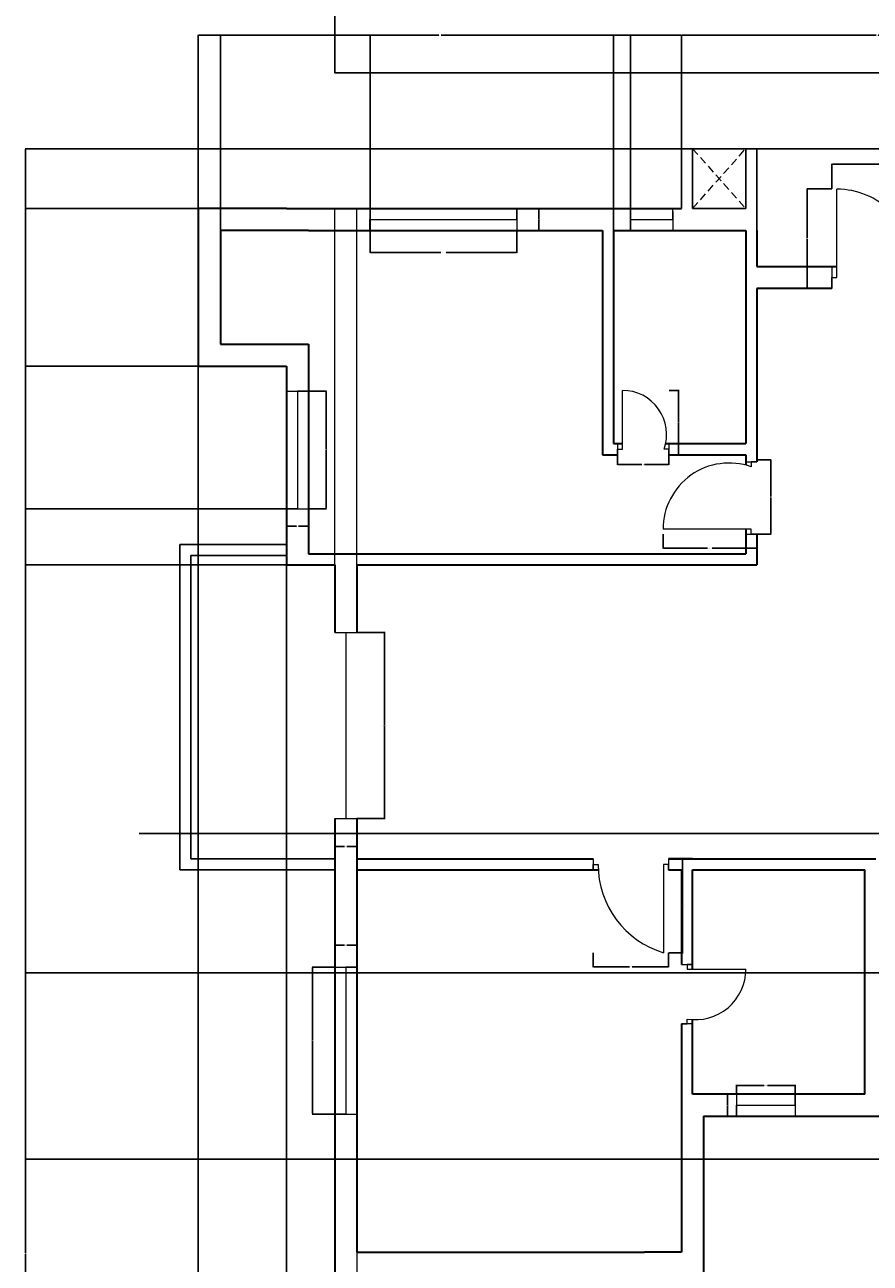
# Model space of a CAD drawing. Units: inches. Extents: x 2296 to 3812, y -1531 to 2564.
# Tile 8 of 10: x 3014 to 3360, y 1720 to 2226. Entities that reach past the tile are written whole.
import ezdxf

# ---------------------------------------------------------------- set-up
doc = ezdxf.new("R2010")
doc.units = ezdxf.units.IN
doc.linetypes.add('HIDDEN2', pattern=[4.7625, 3.175, -1.5875])
for name, color, linetype, lineweight in [('A-ANNO-DIMS', 2, 'Continuous', 18), ('A-ANNO-SYMB', 7, 'Continuous', 25), ('A-DOOR', 3, 'Continuous', 18), ('A-FLOR-HRAL', 7, 'Continuous', 25), ('A-GLAZ', 4, 'Continuous', 18), ('A-SECT-PROJ', 8, 'Continuous', 13), ('A-WALL', 7, 'Continuous', 35), ('A-WALL-HIDN', 8, 'HIDDEN2', 18)]:
    doc.layers.add(name, color=color, linetype=linetype, lineweight=lineweight)
doc.styles.get("Standard").update_dxf_attribs({"font": 'arial.ttf'})
doc.dimstyles.get("Standard").update_dxf_attribs({"dimtxt": 0.18, "dimasz": 0.18, "dimexe": 0.18, "dimexo": 0.0625, "dimgap": 0.09, "dimtad": 0, "dimtih": 1, "dimtoh": 1, "dimdec": 4, "dimzin": 0, "dimdsep": 46, "dimtxsty": 'Standard', "dimcen": 0.09, "dimadec": 0, "dimazin": 0, "dimtfac": 1, "dimtdec": 4, "dimtofl": 0, "dimtmove": 0, "dimatfit": 3, "dimfxl": 1, "dimtolj": 1, "dimtzin": 0, "dimarcsym": 0})

# ---------------------------------------------------------------- blocks, each defined once
blk = doc.blocks.new('DOOR-BEDROOM-ENTRY-NW')
for p, q in [((33.75, 29.46), (38.25, 29.46)), ((38.25, 29.46), (36, 29.46)), ((36, 29.46), (36, 27.46)), ((36, 2), (0, 2)), ((33.75, 0), (38.25, 0)), ((36, 0), (36, 2)), ((38.25, 0), (36, 0))]:
    blk.add_line(p, q)
blk.add_arc((27, 2), 27, 70.5334, 180)
blk = doc.blocks.new('DOOR-BATH-24-NW')
for p, q in [((2, 2.25), (2, 26.25)), ((0, 4.5), (0, 0)), ((0, 0), (0, 2.25)), ((0, 2.25), (2, 2.25)), ((21.01, 2.25), (19.01, 2.25)), ((21.01, 4.5), (21.01, 0)), ((21.01, 0), (21.01, 2.25))]:
    blk.add_line(p, q)
blk.add_arc((2, 8.22), 18.03, 340.6613, 90)
blk = doc.blocks.new('DOOR-BALCONY-PAIR-N')
for p, q in [((2, 4.5), (2, 40.5)), ((64.91, 4.5), (64.91, 40.5)), ((0, 9), (0, 0)), ((66.91, 9), (66.91, 0)), ((0, 0), (0, 4.5)), ((0, 4.5), (2, 4.5)), ((66.91, 4.5), (64.91, 4.5)), ((66.91, 0), (66.91, 4.5))]:
    blk.add_line(p, q)
for centre, radius, start, end in [((2, 9.22), 31.28, 359.5901, 90), ((64.41, 9.36), 31.14, 89.0831, 180.6679)]:
    blk.add_arc(centre, radius, start, end)
blk = doc.blocks.new('DOOR-BEDROOM-36-WN')
for p, q in [((0, 38.25), (0, 33.75)), ((0, 33.75), (0, 36)), ((0, 36), (2, 36)), ((30.77, 36), (28.77, 36)), ((28.77, 36), (28.77, 0)), ((30.77, 38.25), (30.77, 33.75)), ((30.77, 33.75), (30.77, 36))]:
    blk.add_line(p, q)
blk.add_arc((39.59, 36), 37.59, 180, 253.2783)
blk = doc.blocks.new('DOOR-BATH-24-WN')
for p, q in [((0, 24.31), (4.5, 24.31)), ((4.5, 24.31), (2.25, 24.31)), ((2.25, 24.31), (2.25, 22.31)), ((2.25, 22.31), (26.25, 22.31)), ((2.25, 0), (2.25, 2)), ((4.5, 0), (0, 0)), ((0, 0), (2.25, 0))]:
    blk.add_line(p, q)
blk.add_arc((5.66, 22.31), 20.59, 260.4824, 0)
blk = doc.blocks.new('WIN-60-BEDROOM-N')
for p, q in [((0, 9), (0, 0)), ((60, 4.5), (60, 9)), ((60, 9), (60, 0)), ((0, 0), (0, 4.5)), ((0, 4.5), (60, 4.5)), ((60, 4.5), (60, 4.5))]:
    blk.add_line(p, q)
blk = doc.blocks.new('WIN-24-SHAFT-N')
for p, q in [((0, 9), (0, 0)), ((24, 4.5), (24, 9)), ((24, 9), (24, 9)), ((24, 9), (24, 0)), ((0, 0), (0, 4.5)), ((0, 4.5), (24, 4.5))]:
    blk.add_line(p, q)
blk = doc.blocks.new('WIN-60-JAMB-B')
for p, q in [((0, 60), (9, 60)), ((9, 60), (4.5, 60)), ((4.5, 60), (4.5, 0)), ((4.5, 0), (0, 0)), ((0, 0), (9, 0))]:
    blk.add_line(p, q)
blk = doc.blocks.new('WIN-17-VENT')
for p, q in [((0, 9), (0, 0)), ((17.26, 4.5), (17.26, 9)), ((17.26, 7.76), (17.26, 0)), ((0, 0), (0, 4.5)), ((0, 4.5), (0, 4.5)), ((0, 4.5), (17.26, 4.5))]:
    blk.add_line(p, q)
blk = doc.blocks.new('WIN-48-BEDROOM-NW')
for p, q in [((0, 48), (9, 48)), ((9, 48), (4.5, 48)), ((4.5, 48), (4.5, 0)), ((4.5, 0), (0, 0)), ((0, 0), (9, 0))]:
    blk.add_line(p, q)
blk = doc.blocks.new('GLAZ-BALCONY-N')
for p, q in [((0, 75.98), (9, 75.98)), ((4.5, 75.98), (4.5, 0)), ((0, 0), (9, 0))]:
    blk.add_line(p, q)
blk = doc.blocks.new('*D57')
at = {"layer": 'A-ANNO-DIMS', "color": 0, "lineweight": -2, "transparency": 16777216}
for p, q in [((3274.91, 2017.68), (3274.91, 2011.83)), ((3313.16, 2017.68), (3313.16, 2011.83)), ((3275.09, 2012.01), (3293.1, 2012.01)), ((3312.98, 2012.01), (3294.97, 2012.01))]:
    blk.add_line(p, q, dxfattribs=at)
at = {"layer": 'A-ANNO-DIMS', "color": 0, "transparency": 16777216}
for points in [[(3275.09, 2012.04), (3275.09, 2011.98), (3274.91, 2012.01)], [(3312.98, 2012.04), (3312.98, 2011.98), (3313.16, 2012.01)]]:
    blk.add_solid(points, dxfattribs=at)
at = {"layer": 'Defpoints', "color": 0, "transparency": 16777216}
for p in [(3274.91, 2017.75), (3313.16, 2017.75), (3313.16, 2012.01)]:
    blk.add_point(p, dxfattribs=at)
at = {"layer": 'A-ANNO-DIMS', "color": 0, "transparency": 16777216, "insert": (3294.03, 2012.01), "char_height": 0.18, "attachment_point": 5}
blk.add_mtext('\\A1;DOOR 38 TYP.', dxfattribs=at)
blk = doc.blocks.new('*D58')
at = {"layer": 'A-ANNO-DIMS', "color": 0, "lineweight": -2, "transparency": 16777216}
for p, q in [((3313.22, 2048.12), (3319.08, 2048.12)), ((3318.9, 2047.94), (3318.9, 2033.12)), ((3318.9, 2017.93), (3318.9, 2032.75)), ((3313.22, 2017.75), (3319.08, 2017.75))]:
    blk.add_line(p, q, dxfattribs=at)
at = {"layer": 'A-ANNO-DIMS', "color": 0, "transparency": 16777216}
for points in [[(3318.87, 2047.94), (3318.93, 2047.94), (3318.9, 2048.12)], [(3318.87, 2017.93), (3318.93, 2017.93), (3318.9, 2017.75)]]:
    blk.add_solid(points, dxfattribs=at)
at = {"layer": 'Defpoints', "color": 0, "transparency": 16777216}
for p in [(3313.16, 2048.12), (3318.9, 2048.12), (3313.16, 2017.75)]:
    blk.add_point(p, dxfattribs=at)
at = {"layer": 'A-ANNO-DIMS', "color": 0, "transparency": 16777216, "insert": (3318.9, 2032.93), "char_height": 0.18, "attachment_point": 5}
blk.add_mtext('\\A1;30 TYP.', dxfattribs=at)
blk = doc.blocks.new('*D59')
at = {"layer": 'A-ANNO-DIMS', "color": 0, "lineweight": -2, "transparency": 16777216}
for p, q in [((3277.39, 2076.41), (3281.44, 2076.41)), ((3281.26, 2076.23), (3281.26, 2063.47)), ((3281.26, 2050.34), (3281.26, 2063.1)), ((3277.39, 2050.16), (3281.44, 2050.16))]:
    blk.add_line(p, q, dxfattribs=at)
at = {"layer": 'A-ANNO-DIMS', "color": 0, "transparency": 16777216}
for points in [[(3281.23, 2076.23), (3281.29, 2076.23), (3281.26, 2076.41)], [(3281.23, 2050.34), (3281.29, 2050.34), (3281.26, 2050.16)]]:
    blk.add_solid(points, dxfattribs=at)
at = {"layer": 'Defpoints', "color": 0, "transparency": 16777216}
for p in [(3277.33, 2076.41), (3281.26, 2076.41), (3277.33, 2050.16)]:
    blk.add_point(p, dxfattribs=at)
at = {"layer": 'A-ANNO-DIMS', "color": 0, "transparency": 16777216, "insert": (3281.26, 2063.28), "char_height": 0.18, "attachment_point": 5}
blk.add_mtext('\\A1;BATH DOOR 26 TYP.', dxfattribs=at)
blk = doc.blocks.new('*D60')
at = {"layer": 'A-ANNO-DIMS', "color": 0, "lineweight": -2, "transparency": 16777216}
for p, q in [((3256.31, 2050.1), (3256.31, 2046.04)), ((3277.33, 2050.1), (3277.33, 2046.04)), ((3256.49, 2046.22), (3266.29, 2046.22)), ((3277.15, 2046.22), (3267.35, 2046.22))]:
    blk.add_line(p, q, dxfattribs=at)
at = {"layer": 'A-ANNO-DIMS', "color": 0, "transparency": 16777216}
for points in [[(3256.49, 2046.25), (3256.49, 2046.19), (3256.31, 2046.22)], [(3277.15, 2046.25), (3277.15, 2046.19), (3277.33, 2046.22)]]:
    blk.add_solid(points, dxfattribs=at)
at = {"layer": 'Defpoints', "color": 0, "transparency": 16777216}
for p in [(3256.31, 2050.16), (3277.33, 2050.16), (3277.33, 2046.22)]:
    blk.add_point(p, dxfattribs=at)
at = {"layer": 'A-ANNO-DIMS', "color": 0, "transparency": 16777216, "insert": (3266.82, 2046.22), "char_height": 0.18, "attachment_point": 5}
blk.add_mtext('\\A1;21 TYP.', dxfattribs=at)
blk = doc.blocks.new('*D63')
at = {"layer": 'A-ANNO-DIMS', "color": 0, "lineweight": -2, "transparency": 16777216}
for p, q in [((3343.86, 2158.72), (3343.86, 2168.88)), ((3344.04, 2168.7), (3376.46, 2168.7)), ((3410.59, 2168.7), (3378.17, 2168.7)), ((3410.77, 2158.72), (3410.77, 2168.88))]:
    blk.add_line(p, q, dxfattribs=at)
at = {"layer": 'A-ANNO-DIMS', "color": 0, "transparency": 16777216}
for points in [[(3344.04, 2168.73), (3344.04, 2168.67), (3343.86, 2168.7)], [(3410.59, 2168.73), (3410.59, 2168.67), (3410.77, 2168.7)]]:
    blk.add_solid(points, dxfattribs=at)
at = {"layer": 'Defpoints', "color": 0, "transparency": 16777216}
for p in [(3410.77, 2168.7), (3343.86, 2158.66), (3410.77, 2158.66)]:
    blk.add_point(p, dxfattribs=at)
at = {"layer": 'A-ANNO-DIMS', "color": 0, "transparency": 16777216, "insert": (3377.32, 2168.7), "char_height": 0.18, "attachment_point": 5}
blk.add_mtext('\\A1;PAIR 67 TYP.', dxfattribs=at)
blk = doc.blocks.new('*D64')
at = {"layer": 'A-ANNO-DIMS', "color": 0, "lineweight": -2, "transparency": 16777216}
for p, q in [((3343.8, 2158.66), (3333.64, 2158.66)), ((3333.82, 2158.48), (3333.82, 2138.53)), ((3333.82, 2118.21), (3333.82, 2138.16)), ((3343.8, 2118.03), (3333.64, 2118.03))]:
    blk.add_line(p, q, dxfattribs=at)
at = {"layer": 'A-ANNO-DIMS', "color": 0, "transparency": 16777216}
for points in [[(3333.79, 2158.48), (3333.85, 2158.48), (3333.82, 2158.66)], [(3333.79, 2118.21), (3333.85, 2118.21), (3333.82, 2118.03)]]:
    blk.add_solid(points, dxfattribs=at)
at = {"layer": 'Defpoints', "color": 0, "transparency": 16777216}
for p in [(3333.82, 2158.66), (3343.86, 2158.66), (3343.86, 2118.03)]:
    blk.add_point(p, dxfattribs=at)
at = {"layer": 'A-ANNO-DIMS', "color": 0, "transparency": 16777216, "insert": (3333.82, 2138.34), "char_height": 0.18, "attachment_point": 5}
blk.add_mtext('\\A1;41 TYP.', dxfattribs=at)
blk = doc.blocks.new('*D69')
at = {"layer": 'A-ANNO-DIMS', "color": 0, "lineweight": -2, "transparency": 16777216}
for p, q in [((3277.21, 1885.16), (3283.07, 1885.16)), ((3282.89, 1884.98), (3282.89, 1866.22)), ((3282.89, 1847.09), (3282.89, 1865.85)), ((3277.21, 1846.91), (3283.07, 1846.91))]:
    blk.add_line(p, q, dxfattribs=at)
at = {"layer": 'A-ANNO-DIMS', "color": 0, "transparency": 16777216}
for points in [[(3282.86, 1884.98), (3282.92, 1884.98), (3282.89, 1885.16)], [(3282.86, 1847.09), (3282.92, 1847.09), (3282.89, 1846.91)]]:
    blk.add_solid(points, dxfattribs=at)
at = {"layer": 'Defpoints', "color": 0, "transparency": 16777216}
for p in [(3277.15, 1885.16), (3282.89, 1885.16), (3277.15, 1846.91)]:
    blk.add_point(p, dxfattribs=at)
at = {"layer": 'A-ANNO-DIMS', "color": 0, "transparency": 16777216, "insert": (3282.89, 1866.03), "char_height": 0.18, "attachment_point": 5}
blk.add_mtext('\\A1;DOOR 38 TYP.', dxfattribs=at)
blk = doc.blocks.new('*D70')
at = {"layer": 'A-ANNO-DIMS', "color": 0, "lineweight": -2, "transparency": 16777216}
for p, q in [((3246.37, 1846.85), (3246.37, 1840.99)), ((3277.15, 1846.85), (3277.15, 1840.99)), ((3246.55, 1841.17), (3261.23, 1841.17)), ((3276.97, 1841.17), (3262.29, 1841.17))]:
    blk.add_line(p, q, dxfattribs=at)
at = {"layer": 'A-ANNO-DIMS', "color": 0, "transparency": 16777216}
for points in [[(3246.55, 1841.2), (3246.55, 1841.14), (3246.37, 1841.17)], [(3276.97, 1841.2), (3276.97, 1841.14), (3277.15, 1841.17)]]:
    blk.add_solid(points, dxfattribs=at)
at = {"layer": 'Defpoints', "color": 0, "transparency": 16777216}
for p in [(3246.37, 1846.91), (3277.15, 1846.91), (3277.15, 1841.17)]:
    blk.add_point(p, dxfattribs=at)
at = {"layer": 'A-ANNO-DIMS', "color": 0, "transparency": 16777216, "insert": (3261.76, 1841.17), "char_height": 0.18, "attachment_point": 5}
blk.add_mtext('\\A1;31 TYP.', dxfattribs=at)
blk = doc.blocks.new('*D101')
at = {"layer": 'A-ANNO-DIMS', "color": 0, "lineweight": -2, "transparency": 16777216}
for p, q in [((3155.26, 2141.6), (3155.26, 2132.48)), ((3215.26, 2141.6), (3215.26, 2132.48)), ((3155.44, 2132.66), (3184.14, 2132.66)), ((3215.08, 2132.66), (3186.38, 2132.66))]:
    blk.add_line(p, q, dxfattribs=at)
at = {"layer": 'A-ANNO-DIMS', "color": 0, "transparency": 16777216}
for points in [[(3155.44, 2132.69), (3155.44, 2132.63), (3155.26, 2132.66)], [(3215.08, 2132.69), (3215.08, 2132.63), (3215.26, 2132.66)]]:
    blk.add_solid(points, dxfattribs=at)
at = {"layer": 'Defpoints', "color": 0, "transparency": 16777216}
for p in [(3155.26, 2141.66), (3215.26, 2141.66), (3215.26, 2132.66)]:
    blk.add_point(p, dxfattribs=at)
at = {"layer": 'A-ANNO-DIMS', "color": 0, "transparency": 16777216, "insert": (3185.26, 2132.66), "char_height": 0.18, "attachment_point": 5}
blk.add_mtext('\\A1;WINDOW 60 TYP.', dxfattribs=at)
blk = doc.blocks.new('*D102')
at = {"layer": 'A-ANNO-DIMS', "color": 0, "lineweight": -2, "transparency": 16777216}
for p, q in [((3215.32, 2150.66), (3224.44, 2150.66)), ((3224.26, 2150.48), (3224.26, 2146.34)), ((3224.26, 2141.84), (3224.26, 2145.98)), ((3215.32, 2141.66), (3224.44, 2141.66))]:
    blk.add_line(p, q, dxfattribs=at)
at = {"layer": 'A-ANNO-DIMS', "color": 0, "transparency": 16777216}
for points in [[(3224.23, 2150.48), (3224.29, 2150.48), (3224.26, 2150.66)], [(3224.23, 2141.84), (3224.29, 2141.84), (3224.26, 2141.66)]]:
    blk.add_solid(points, dxfattribs=at)
at = {"layer": 'Defpoints', "color": 0, "transparency": 16777216}
for p in [(3215.26, 2150.66), (3224.26, 2150.66), (3215.26, 2141.66)]:
    blk.add_point(p, dxfattribs=at)
at = {"layer": 'A-ANNO-DIMS', "color": 0, "transparency": 16777216, "insert": (3224.26, 2146.16), "char_height": 0.18, "attachment_point": 5}
blk.add_mtext('\\A1;9 TYP.', dxfattribs=at)
blk = doc.blocks.new('*D109')
at = {"layer": 'A-ANNO-DIMS', "color": 0, "lineweight": -2, "transparency": 16777216}
for p, q in [((3304.87, 1789.22), (3304.87, 1792.94)), ((3305.05, 1792.76), (3316.22, 1792.76)), ((3328.7, 1792.76), (3317.53, 1792.76)), ((3328.88, 1789.22), (3328.88, 1792.94))]:
    blk.add_line(p, q, dxfattribs=at)
at = {"layer": 'A-ANNO-DIMS', "color": 0, "transparency": 16777216}
for points in [[(3305.05, 1792.79), (3305.05, 1792.73), (3304.87, 1792.76)], [(3328.7, 1792.79), (3328.7, 1792.73), (3328.88, 1792.76)]]:
    blk.add_solid(points, dxfattribs=at)
at = {"layer": 'Defpoints', "color": 0, "transparency": 16777216}
for p in [(3328.88, 1792.76), (3304.87, 1789.16), (3328.88, 1789.16)]:
    blk.add_point(p, dxfattribs=at)
at = {"layer": 'A-ANNO-DIMS', "color": 0, "transparency": 16777216, "insert": (3316.88, 1792.76), "char_height": 0.18, "attachment_point": 5}
blk.add_mtext('\\A1;V 24 TYP.', dxfattribs=at)
blk = doc.blocks.new('*D110')
at = {"layer": 'A-ANNO-DIMS', "color": 0, "lineweight": -2, "transparency": 16777216}
for p, q in [((3304.81, 1789.16), (3301.09, 1789.16)), ((3301.27, 1788.98), (3301.27, 1784.84)), ((3301.27, 1780.34), (3301.27, 1784.48)), ((3304.81, 1780.16), (3301.09, 1780.16))]:
    blk.add_line(p, q, dxfattribs=at)
at = {"layer": 'A-ANNO-DIMS', "color": 0, "transparency": 16777216}
for points in [[(3301.24, 1788.98), (3301.3, 1788.98), (3301.27, 1789.16)], [(3301.24, 1780.34), (3301.3, 1780.34), (3301.27, 1780.16)]]:
    blk.add_solid(points, dxfattribs=at)
at = {"layer": 'Defpoints', "color": 0, "transparency": 16777216}
for p in [(3301.27, 1789.16), (3304.87, 1789.16), (3304.87, 1780.16)]:
    blk.add_point(p, dxfattribs=at)
at = {"layer": 'A-ANNO-DIMS', "color": 0, "transparency": 16777216, "insert": (3301.27, 1784.66), "char_height": 0.18, "attachment_point": 5}
blk.add_mtext('\\A1;9 TYP.', dxfattribs=at)
blk = doc.blocks.new('*D111')
at = {"layer": 'A-ANNO-DIMS', "color": 0, "lineweight": -2, "transparency": 16777216}
for p, q in [((3140.78, 1841.04), (3131.66, 1841.04)), ((3131.84, 1840.86), (3131.84, 1811.23)), ((3131.84, 1781.22), (3131.84, 1810.86)), ((3140.78, 1781.04), (3131.66, 1781.04))]:
    blk.add_line(p, q, dxfattribs=at)
at = {"layer": 'A-ANNO-DIMS', "color": 0, "transparency": 16777216}
for points in [[(3131.81, 1840.86), (3131.87, 1840.86), (3131.84, 1841.04)], [(3131.81, 1781.22), (3131.87, 1781.22), (3131.84, 1781.04)]]:
    blk.add_solid(points, dxfattribs=at)
at = {"layer": 'Defpoints', "color": 0, "transparency": 16777216}
for p in [(3131.84, 1841.04), (3140.84, 1841.04), (3140.84, 1781.04)]:
    blk.add_point(p, dxfattribs=at)
at = {"layer": 'A-ANNO-DIMS', "color": 0, "transparency": 16777216, "insert": (3131.84, 1811.04), "char_height": 0.18, "attachment_point": 5}
blk.add_mtext('\\A1;WINDOW 60 TYP.', dxfattribs=at)
blk = doc.blocks.new('*D112')
at = {"layer": 'A-ANNO-DIMS', "color": 0, "lineweight": -2, "transparency": 16777216}
for p, q in [((3140.84, 1841.11), (3140.84, 1850.22)), ((3141.02, 1850.04), (3144.88, 1850.04)), ((3149.66, 1850.04), (3145.8, 1850.04)), ((3149.84, 1841.11), (3149.84, 1850.22))]:
    blk.add_line(p, q, dxfattribs=at)
at = {"layer": 'A-ANNO-DIMS', "color": 0, "transparency": 16777216}
for points in [[(3141.02, 1850.07), (3141.02, 1850.01), (3140.84, 1850.04)], [(3149.66, 1850.07), (3149.66, 1850.01), (3149.84, 1850.04)]]:
    blk.add_solid(points, dxfattribs=at)
at = {"layer": 'Defpoints', "color": 0, "transparency": 16777216}
for p in [(3149.84, 1850.04), (3140.84, 1841.04), (3149.84, 1841.04)]:
    blk.add_point(p, dxfattribs=at)
at = {"layer": 'A-ANNO-DIMS', "color": 0, "transparency": 16777216, "insert": (3145.34, 1850.04), "char_height": 0.18, "attachment_point": 5}
blk.add_mtext('\\A1;9 TYP.', dxfattribs=at)
blk = doc.blocks.new('*D121')
at = {"layer": 'A-ANNO-DIMS', "color": 0, "lineweight": -2, "transparency": 16777216}
for p, q in [((3130.22, 2076.12), (3137.54, 2076.12)), ((3137.36, 2075.94), (3137.36, 2052.31)), ((3137.36, 2028.3), (3137.36, 2051.94)), ((3130.22, 2028.12), (3137.54, 2028.12))]:
    blk.add_line(p, q, dxfattribs=at)
at = {"layer": 'A-ANNO-DIMS', "color": 0, "transparency": 16777216}
for points in [[(3137.33, 2075.94), (3137.39, 2075.94), (3137.36, 2076.12)], [(3137.33, 2028.3), (3137.39, 2028.3), (3137.36, 2028.12)]]:
    blk.add_solid(points, dxfattribs=at)
at = {"layer": 'Defpoints', "color": 0, "transparency": 16777216}
for p in [(3130.16, 2076.12), (3137.36, 2076.12), (3130.16, 2028.12)]:
    blk.add_point(p, dxfattribs=at)
at = {"layer": 'A-ANNO-DIMS', "color": 0, "transparency": 16777216, "insert": (3137.36, 2052.12), "char_height": 0.18, "attachment_point": 5}
blk.add_mtext('\\A1;WINDOW 48 TYP.', dxfattribs=at)
blk = doc.blocks.new('*D122')
at = {"layer": 'A-ANNO-DIMS', "color": 0, "lineweight": -2, "transparency": 16777216}
for p, q in [((3121.16, 2028.06), (3121.16, 2020.74)), ((3130.16, 2028.06), (3130.16, 2020.74)), ((3121.34, 2020.92), (3125.2, 2020.92)), ((3129.98, 2020.92), (3126.12, 2020.92))]:
    blk.add_line(p, q, dxfattribs=at)
at = {"layer": 'A-ANNO-DIMS', "color": 0, "transparency": 16777216}
for points in [[(3121.34, 2020.95), (3121.34, 2020.89), (3121.16, 2020.92)], [(3129.98, 2020.95), (3129.98, 2020.89), (3130.16, 2020.92)]]:
    blk.add_solid(points, dxfattribs=at)
at = {"layer": 'Defpoints', "color": 0, "transparency": 16777216}
for p in [(3121.16, 2028.12), (3130.16, 2028.12), (3130.16, 2020.92)]:
    blk.add_point(p, dxfattribs=at)
at = {"layer": 'A-ANNO-DIMS', "color": 0, "transparency": 16777216, "insert": (3125.66, 2020.92), "char_height": 0.18, "attachment_point": 5}
blk.add_mtext('\\A1;9 TYP.', dxfattribs=at)
blk = doc.blocks.new('*D125')
at = {"layer": 'A-ANNO-DIMS', "color": 0, "lineweight": -2, "transparency": 16777216}
for p, q in [((3149.9, 1977.62), (3161.42, 1977.62)), ((3161.24, 1977.44), (3161.24, 1939.81)), ((3161.24, 1901.82), (3161.24, 1939.44)), ((3149.9, 1901.64), (3161.42, 1901.64))]:
    blk.add_line(p, q, dxfattribs=at)
at = {"layer": 'A-ANNO-DIMS', "color": 0, "transparency": 16777216}
for points in [[(3161.21, 1977.44), (3161.27, 1977.44), (3161.24, 1977.62)], [(3161.21, 1901.82), (3161.27, 1901.82), (3161.24, 1901.64)]]:
    blk.add_solid(points, dxfattribs=at)
at = {"layer": 'Defpoints', "color": 0, "transparency": 16777216}
for p in [(3149.84, 1977.62), (3161.24, 1977.62), (3149.84, 1901.64)]:
    blk.add_point(p, dxfattribs=at)
at = {"layer": 'A-ANNO-DIMS', "color": 0, "transparency": 16777216, "insert": (3161.24, 1939.63), "char_height": 0.18, "attachment_point": 5}
blk.add_mtext('\\A1;GLAZING 76 TYP.', dxfattribs=at)
blk = doc.blocks.new('*D126')
at = {"layer": 'A-ANNO-DIMS', "color": 0, "lineweight": -2, "transparency": 16777216}
for p, q in [((3140.84, 1901.57), (3140.84, 1890.06)), ((3149.84, 1901.57), (3149.84, 1890.06)), ((3141.02, 1890.24), (3144.88, 1890.24)), ((3149.66, 1890.24), (3145.8, 1890.24))]:
    blk.add_line(p, q, dxfattribs=at)
at = {"layer": 'A-ANNO-DIMS', "color": 0, "transparency": 16777216}
for points in [[(3141.02, 1890.27), (3141.02, 1890.21), (3140.84, 1890.24)], [(3149.66, 1890.27), (3149.66, 1890.21), (3149.84, 1890.24)]]:
    blk.add_solid(points, dxfattribs=at)
at = {"layer": 'Defpoints', "color": 0, "transparency": 16777216}
for p in [(3140.84, 1901.64), (3149.84, 1901.64), (3149.84, 1890.24)]:
    blk.add_point(p, dxfattribs=at)
at = {"layer": 'A-ANNO-DIMS', "color": 0, "transparency": 16777216, "insert": (3145.34, 1890.24), "char_height": 0.18, "attachment_point": 5}
blk.add_mtext('\\A1;9 TYP.', dxfattribs=at)
blk = doc.blocks.new('*D130')
at = {"layer": 'A-ANNO-DIMS', "color": 0, "lineweight": -2, "transparency": 16777216}
for p, q in [((3313.1, 2175.03), (3014.48, 2175.03)), ((3014.66, 2174.85), (3014.66, 1724.41)), ((3014.66, 1273.61), (3014.66, 1724.05)), ((3319.28, 1273.43), (3014.48, 1273.43))]:
    blk.add_line(p, q, dxfattribs=at)
at = {"layer": 'A-ANNO-DIMS', "color": 0, "transparency": 16777216}
for points in [[(3014.63, 2174.85), (3014.69, 2174.85), (3014.66, 2175.03)], [(3014.63, 1273.61), (3014.69, 1273.61), (3014.66, 1273.43)]]:
    blk.add_solid(points, dxfattribs=at)
at = {"layer": 'Defpoints', "color": 0, "transparency": 16777216}
for p in [(3014.66, 2175.03), (3313.16, 2175.03), (3319.34, 1273.43)]:
    blk.add_point(p, dxfattribs=at)
at = {"layer": 'A-ANNO-DIMS', "color": 0, "transparency": 16777216, "insert": (3014.66, 1724.23), "char_height": 0.18, "attachment_point": 5}
blk.add_mtext('\\A1;901.6', dxfattribs=at)
blk = doc.blocks.new('*D131')
at = {"layer": 'A-ANNO-DIMS', "color": 0, "lineweight": -2, "transparency": 16777216}
for p, q in [((3085.16, 2150.72), (3085.16, 2221.56)), ((3085.34, 2221.38), (3183.38, 2221.38)), ((3282.33, 2221.38), (3184.29, 2221.38)), ((3282.51, 2175.09), (3282.51, 2221.56))]:
    blk.add_line(p, q, dxfattribs=at)
at = {"layer": 'A-ANNO-DIMS', "color": 0, "transparency": 16777216}
for points in [[(3085.34, 2221.41), (3085.34, 2221.35), (3085.16, 2221.38)], [(3282.33, 2221.41), (3282.33, 2221.35), (3282.51, 2221.38)]]:
    blk.add_solid(points, dxfattribs=at)
at = {"layer": 'Defpoints', "color": 0, "transparency": 16777216}
for p in [(3282.51, 2221.38), (3282.51, 2175.03), (3085.16, 2150.66)]:
    blk.add_point(p, dxfattribs=at)
at = {"layer": 'A-ANNO-DIMS', "color": 0, "transparency": 16777216, "insert": (3183.83, 2221.38), "char_height": 0.18, "attachment_point": 5}
blk.add_mtext('\\A1;197.35', dxfattribs=at)
blk = doc.blocks.new('*D132')
at = {"layer": 'A-ANNO-DIMS', "color": 0, "lineweight": -2, "transparency": 16777216}
for p, q in [((3282.51, 2175.09), (3282.51, 2221.56)), ((3282.69, 2221.38), (3361.88, 2221.38)), ((3441.98, 2221.38), (3362.79, 2221.38)), ((3442.16, 2175.09), (3442.16, 2221.56))]:
    blk.add_line(p, q, dxfattribs=at)
at = {"layer": 'A-ANNO-DIMS', "color": 0, "transparency": 16777216}
for points in [[(3282.69, 2221.41), (3282.69, 2221.35), (3282.51, 2221.38)], [(3441.98, 2221.41), (3441.98, 2221.35), (3442.16, 2221.38)]]:
    blk.add_solid(points, dxfattribs=at)
at = {"layer": 'Defpoints', "color": 0, "transparency": 16777216}
for p in [(3442.16, 2221.38), (3282.51, 2175.03), (3442.16, 2175.03)]:
    blk.add_point(p, dxfattribs=at)
at = {"layer": 'A-ANNO-DIMS', "color": 0, "transparency": 16777216, "insert": (3362.33, 2221.38), "char_height": 0.18, "attachment_point": 5}
blk.add_mtext('\\A1;159.65', dxfattribs=at)
blk = doc.blocks.new('*D141')
at = {"layer": 'A-ANNO-DIMS', "color": 0, "lineweight": -2, "transparency": 16777216}
for p, q in [((3452.27, 1838.66), (3014.48, 1838.66)), ((3014.66, 1838.48), (3014.66, 1800.83)), ((3014.66, 1762.81), (3014.66, 1800.46)), ((3452.27, 1762.63), (3014.48, 1762.63))]:
    blk.add_line(p, q, dxfattribs=at)
at = {"layer": 'A-ANNO-DIMS', "color": 0, "transparency": 16777216}
for points in [[(3014.63, 1838.48), (3014.69, 1838.48), (3014.66, 1838.66)], [(3014.63, 1762.81), (3014.69, 1762.81), (3014.66, 1762.63)]]:
    blk.add_solid(points, dxfattribs=at)
at = {"layer": 'Defpoints', "color": 0, "transparency": 16777216}
for p in [(3014.66, 1838.66), (3452.33, 1838.66), (3452.33, 1762.63)]:
    blk.add_point(p, dxfattribs=at)
at = {"layer": 'A-ANNO-DIMS', "color": 0, "transparency": 16777216, "insert": (3014.66, 1800.64), "char_height": 0.18, "attachment_point": 5}
blk.add_mtext('\\A1;76.03', dxfattribs=at)
blk = doc.blocks.new('*D142')
at = {"layer": 'A-ANNO-DIMS', "color": 0, "lineweight": -2, "transparency": 16777216}
for p, q in [((3094.16, 2141.72), (3094.16, 2221.56)), ((3094.34, 2221.38), (3124.4, 2221.38)), ((3155.08, 2221.38), (3125.01, 2221.38)), ((3155.26, 2141.72), (3155.26, 2221.56))]:
    blk.add_line(p, q, dxfattribs=at)
at = {"layer": 'A-ANNO-DIMS', "color": 0, "transparency": 16777216}
for points in [[(3094.34, 2221.41), (3094.34, 2221.35), (3094.16, 2221.38)], [(3155.08, 2221.41), (3155.08, 2221.35), (3155.26, 2221.38)]]:
    blk.add_solid(points, dxfattribs=at)
at = {"layer": 'Defpoints', "color": 0, "transparency": 16777216}
for p in [(3155.26, 2221.38), (3094.16, 2141.66), (3155.26, 2141.66)]:
    blk.add_point(p, dxfattribs=at)
at = {"layer": 'A-ANNO-DIMS', "color": 0, "transparency": 16777216, "insert": (3124.71, 2221.38), "char_height": 0.18, "attachment_point": 5}
blk.add_mtext('\\A1;61.1', dxfattribs=at)
blk = doc.blocks.new('*D143')
at = {"layer": 'A-ANNO-DIMS', "color": 0, "lineweight": -2, "transparency": 16777216}
for p, q in [((3085.16, 2086.2), (3085.16, 1226.9)), ((3121.16, 2086.2), (3121.16, 1226.9)), ((3085.34, 1227.08), (3102.94, 1227.08)), ((3120.98, 1227.08), (3103.38, 1227.08))]:
    blk.add_line(p, q, dxfattribs=at)
at = {"layer": 'A-ANNO-DIMS', "color": 0, "transparency": 16777216}
for points in [[(3085.34, 1227.11), (3085.34, 1227.05), (3085.16, 1227.08)], [(3120.98, 1227.11), (3120.98, 1227.05), (3121.16, 1227.08)]]:
    blk.add_solid(points, dxfattribs=at)
at = {"layer": 'Defpoints', "color": 0, "transparency": 16777216}
for p in [(3085.16, 2086.26), (3121.16, 2086.26), (3121.16, 1227.08)]:
    blk.add_point(p, dxfattribs=at)
at = {"layer": 'A-ANNO-DIMS', "color": 0, "transparency": 16777216, "insert": (3103.16, 1227.08), "char_height": 0.18, "attachment_point": 5}
blk.add_mtext('\\A1;36', dxfattribs=at)
blk = doc.blocks.new('*D144')
at = {"layer": 'A-ANNO-DIMS', "color": 0, "lineweight": -2, "transparency": 16777216}
for p, q in [((3085.1, 2150.66), (3014.48, 2150.66)), ((3014.66, 2150.48), (3014.66, 2118.64)), ((3014.66, 2086.44), (3014.66, 2118.28)), ((3085.1, 2086.26), (3014.48, 2086.26))]:
    blk.add_line(p, q, dxfattribs=at)
at = {"layer": 'A-ANNO-DIMS', "color": 0, "transparency": 16777216}
for points in [[(3014.63, 2150.48), (3014.69, 2150.48), (3014.66, 2150.66)], [(3014.63, 2086.44), (3014.69, 2086.44), (3014.66, 2086.26)]]:
    blk.add_solid(points, dxfattribs=at)
at = {"layer": 'Defpoints', "color": 0, "transparency": 16777216}
for p in [(3014.66, 2150.66), (3085.16, 2150.66), (3085.16, 2086.26)]:
    blk.add_point(p, dxfattribs=at)
at = {"layer": 'A-ANNO-DIMS', "color": 0, "transparency": 16777216, "insert": (3014.66, 2118.46), "char_height": 0.18, "attachment_point": 5}
blk.add_mtext('\\A1;64.39', dxfattribs=at)
blk = doc.blocks.new('*D145')
at = {"layer": 'A-ANNO-DIMS', "color": 0, "lineweight": -2, "transparency": 16777216}
for p, q in [((3254.66, 2141.72), (3254.66, 2221.56)), ((3254.84, 2221.38), (3257.74, 2221.38)), ((3261.44, 2221.38), (3258.53, 2221.38)), ((3261.62, 2141.72), (3261.62, 2221.56))]:
    blk.add_line(p, q, dxfattribs=at)
at = {"layer": 'A-ANNO-DIMS', "color": 0, "transparency": 16777216}
for points in [[(3254.84, 2221.41), (3254.84, 2221.35), (3254.66, 2221.38)], [(3261.44, 2221.41), (3261.44, 2221.35), (3261.62, 2221.38)]]:
    blk.add_solid(points, dxfattribs=at)
at = {"layer": 'Defpoints', "color": 0, "transparency": 16777216}
for p in [(3261.62, 2221.38), (3254.66, 2141.66), (3261.62, 2141.66)]:
    blk.add_point(p, dxfattribs=at)
at = {"layer": 'A-ANNO-DIMS', "color": 0, "transparency": 16777216, "insert": (3258.14, 2221.38), "char_height": 0.18, "attachment_point": 5}
blk.add_mtext('\\A1;6.957', dxfattribs=at)
blk = doc.blocks.new('*D146')
at = {"layer": 'A-ANNO-DIMS', "color": 0, "lineweight": -2, "transparency": 16777216}
for p, q in [((3121.1, 2028.12), (3014.48, 2028.12)), ((3014.66, 2027.94), (3014.66, 2016.82)), ((3014.66, 2005.34), (3014.66, 2016.46)), ((3121.1, 2005.16), (3014.48, 2005.16))]:
    blk.add_line(p, q, dxfattribs=at)
at = {"layer": 'A-ANNO-DIMS', "color": 0, "transparency": 16777216}
for points in [[(3014.63, 2027.94), (3014.69, 2027.94), (3014.66, 2028.12)], [(3014.63, 2005.34), (3014.69, 2005.34), (3014.66, 2005.16)]]:
    blk.add_solid(points, dxfattribs=at)
at = {"layer": 'Defpoints', "color": 0, "transparency": 16777216}
for p in [(3121.16, 2028.12), (3014.66, 2005.16), (3121.16, 2005.16)]:
    blk.add_point(p, dxfattribs=at)
at = {"layer": 'A-ANNO-DIMS', "color": 0, "transparency": 16777216, "insert": (3014.66, 2016.64), "char_height": 0.18, "attachment_point": 5}
blk.add_mtext('\\A1;22.967', dxfattribs=at)
blk = doc.blocks.new('*D159')
at = {"layer": 'A-ANNO-DIMS', "color": 0, "lineweight": -2, "transparency": 16777216}
for p, q in [((3140.84, 2277.72), (3140.84, 2205.81)), ((3597.32, 2277.72), (3597.32, 2205.81)), ((3141.02, 2205.99), (3368.68, 2205.99)), ((3597.14, 2205.99), (3369.48, 2205.99))]:
    blk.add_line(p, q, dxfattribs=at)
at = {"layer": 'A-ANNO-DIMS', "color": 0, "transparency": 16777216}
for points in [[(3141.02, 2206.02), (3141.02, 2205.96), (3140.84, 2205.99)], [(3597.14, 2206.02), (3597.14, 2205.96), (3597.32, 2205.99)]]:
    blk.add_solid(points, dxfattribs=at)
at = {"layer": 'Defpoints', "color": 0, "transparency": 16777216}
for p in [(3140.84, 2277.78), (3597.32, 2277.78), (3597.32, 2205.99)]:
    blk.add_point(p, dxfattribs=at)
at = {"layer": 'A-ANNO-DIMS', "color": 0, "transparency": 16777216, "insert": (3369.08, 2205.99), "char_height": 0.18, "attachment_point": 5}
blk.add_mtext('\\A1;456.5', dxfattribs=at)

msp = doc.modelspace()

# ---------------------------------------------------------------- linework, layer by layer
at = {"layer": 'A-ANNO-SYMB'}
msp.add_line((3061.0144, 1895.5359), (3697.3821, 1895.5359), dxfattribs=at)
at = {"layer": 'A-FLOR-HRAL'}
for p, q in [((3282.5073, 2150.6578), (3282.5073, 2175.0276)), ((3282.5073, 2175.0276), (3287.0073, 2175.0276)), ((3287.0073, 2175.0276), (3287.0073, 2150.6578)), ((3308.6588, 2150.6578), (3308.6588, 2175.0276)), ((3442.1588, 2175.0276), (3308.6588, 2175.0276)), ((3313.1588, 2141.6578), (3313.1588, 2175.0276)), ((3313.1588, 2127.0276), (3313.1588, 2175.0276)), ((3313.1588, 2175.0276), (3442.1588, 2175.0276)), ((3287.0073, 2150.6578), (3308.6588, 2150.6578)), ((3287.0073, 2150.6578), (3308.6588, 2150.6578)), ((3121.1588, 2013.471), (3077.6588, 2013.471)), ((3077.6588, 2013.471), (3077.6588, 1884.8249)), ((3082.1588, 1889.3249), (3082.1588, 2008.971)), ((3082.1588, 2008.971), (3121.1588, 2008.971)), ((3082.1588, 1885.1578), (3082.1588, 1889.3249)), ((3077.6588, 1880.6578), (3077.6588, 1884.8249)), ((3140.8418, 1880.6578), (3077.6588, 1880.6578)), ((3140.8418, 1885.1578), (3082.1588, 1885.1578))]:
    msp.add_line(p, q, dxfattribs=at)
at = {"layer": 'A-SECT-PROJ'}
for p, q in [((3140.8418, 1977.6187), (3140.8418, 2150.6578)), ((3149.8418, 1977.6187), (3149.8418, 2150.6578)), ((3140.8418, 1901.6355), (3140.8418, 1540.9318)), ((3149.8418, 1901.6355), (3149.8418, 1540.9318))]:
    msp.add_line(p, q, dxfattribs=at)
at = {"layer": 'A-WALL'}
for p, q in [((3121.1588, 2150.6578), (3085.1588, 2150.6578)), ((3085.1588, 2150.6578), (3085.1588, 2086.2649)), ((3121.1588, 2150.6578), (3282.5073, 2150.6578)), ((3121.1588, 2150.6578), (3282.5073, 2150.6578)), ((3130.1588, 2141.6578), (3094.1588, 2141.6578)), ((3094.1588, 2141.6578), (3094.1588, 2095.2649)), ((3130.1588, 2141.6578), (3250.1588, 2141.6578)), ((3250.1588, 2141.6578), (3250.1588, 2050.1578)), ((3254.6588, 2141.6578), (3254.6588, 2054.6578)), ((3254.6588, 2141.6578), (3308.6588, 2141.6578)), ((3308.6588, 2141.6578), (3308.6588, 2054.6578)), ((3313.1588, 2141.6578), (3313.1588, 2127.0276)), ((3313.1588, 2127.0276), (3345.86, 2127.0276)), ((3313.1588, 2118.0276), (3313.1588, 2047.2032)), ((3343.86, 2118.0276), (3313.1588, 2118.0276)), ((3094.1588, 2095.2649), (3130.1588, 2095.2649)), ((3130.1588, 2095.2649), (3130.1588, 2009.6578)), ((3085.1588, 2086.2649), (3121.1588, 2086.2649)), ((3121.1588, 2086.2649), (3121.1588, 2005.1578)), ((3121.1588, 2086.2649), (3121.1588, 2005.1578)), ((3254.6588, 2054.6578), (3258.3142, 2054.6578)), ((3275.9556, 2054.6578), (3308.6588, 2054.6578)), ((3250.1588, 2050.1578), (3256.3142, 2050.1578)), ((3277.3264, 2050.1578), (3308.6588, 2050.1578)), ((3308.6588, 2050.1578), (3308.6588, 2045.8898)), ((3308.6588, 2019.7452), (3308.6588, 2009.6578)), ((3313.1588, 2017.7452), (3313.1588, 2005.1578)), ((3130.1588, 2009.6578), (3308.6588, 2009.6578)), ((3121.1588, 2005.1578), (3140.8418, 2005.1578)), ((3140.8418, 2005.1578), (3140.8418, 1977.6187)), ((3149.8418, 2005.1578), (3254.6588, 2005.1578)), ((3149.8418, 2005.1578), (3149.8418, 1977.6187)), ((3254.6588, 2005.1578), (3313.1588, 2005.1578)), ((3140.8418, 1901.6355), (3140.8418, 1540.9318)), ((3149.8418, 1901.6355), (3149.8418, 1724.6578)), ((3149.8418, 1885.1578), (3246.3738, 1885.1578)), ((3149.8418, 1880.6578), (3248.4412, 1880.6578)), ((3149.8418, 1880.6578), (3248.4412, 1880.6578)), ((3286.9894, 1885.1578), (3277.1479, 1885.1578)), ((3277.1479, 1885.1578), (3361.7648, 1885.1578)), ((3277.1479, 1880.6578), (3282.4894, 1880.6578)), ((3277.1479, 1880.6578), (3282.4894, 1880.6578)), ((3282.4894, 1880.6578), (3282.4894, 1842.135)), ((3286.9894, 1840.135), (3286.9894, 1880.6578)), ((3286.9894, 1880.6578), (3357.2648, 1880.6578)), ((3357.2648, 1847.6578), (3357.2648, 1880.6578)), ((3357.2648, 1789.1578), (3357.2648, 1847.6578)), ((3282.4894, 1817.8238), (3282.4894, 1724.6578)), ((3286.9894, 1789.1578), (3286.9894, 1819.5727)), ((3282.4894, 1788.9038), (3282.4894, 1788.9038)), ((3357.2648, 1789.1578), (3286.9894, 1789.1578)), ((3291.4894, 1780.1578), (3366.2648, 1780.1578)), ((3291.4894, 1780.1578), (3291.4894, 1715.6578)), ((3149.8418, 1724.6578), (3267.3064, 1724.6578)), ((3282.4894, 1724.6578), (3267.3064, 1724.6578))]:
    msp.add_line(p, q, dxfattribs=at)
at = {"layer": 'A-WALL-HIDN'}
for p, q in [((3287.0073, 2175.0276), (3308.6588, 2150.6578)), ((3287.0073, 2150.6578), (3308.6588, 2175.0276))]:
    msp.add_line(p, q, dxfattribs=at)

# ---------------------------------------------------------------- block references
at = {"layer": 'A-DOOR'}
for name, p in [('DOOR-BALCONY-PAIR-N', (3343.8604, 2118.028)), ('DOOR-BATH-24-NW', (3256.3144, 2050.158)), ('DOOR-BEDROOM-ENTRY-NW', (3274.9084, 2017.745)), ('DOOR-BEDROOM-36-WN', (3246.3734, 1846.908)), ('DOOR-BATH-24-WN', (3282.4894, 1817.824))]:
    msp.add_blockref(name, p, dxfattribs=at)
at = {"layer": 'A-GLAZ'}
for name, p in [('WIN-60-BEDROOM-N', (3155.2564, 2141.658)), ('WIN-17-VENT', (3261.6164, 2141.658)), ('WIN-48-BEDROOM-NW', (3121.1584, 2028.125)), ('GLAZ-BALCONY-N', (3140.8414, 1901.636)), ('WIN-60-JAMB-B', (3140.8414, 1781.045)), ('WIN-24-SHAFT-N', (3304.8734, 1780.158))]:
    msp.add_blockref(name, p, dxfattribs=at)

# ---------------------------------------------------------------- dimensions: what is measured, and where the dimension line sits
at = {"layer": 'A-ANNO-DIMS'}
for base, p1, p2, override, picture, middle in [((3597.3177, 2205.9928), (3140.8418, 2277.7848), (3597.3177, 2277.7848), {"dimdec": 1, "dimlfac": 1, "dimrnd": 0, "dimzin": 0, "dimdsep": 46, "dimlunit": 2}, '*D159', (3369.0797, 2205.9928)), ((3282.5073, 2221.3776), (3085.1588, 2150.6578), (3282.5073, 2175.0276), {"dimdec": 2, "dimlfac": 1, "dimrnd": 0, "dimzin": 0, "dimdsep": 46, "dimlunit": 2}, '*D131', (3183.833, 2221.3776)), ((3155.2567, 2221.3776), (3094.1588, 2141.6578), (3155.2567, 2141.6578), {"dimdec": 1, "dimlfac": 1, "dimrnd": 0, "dimzin": 0, "dimdsep": 46, "dimlunit": 2}, '*D142', (3124.7077, 2221.3776)), ((3261.6161, 2221.3776), (3254.6588, 2141.6578), (3261.6161, 2141.6578), {"dimdec": 3, "dimlfac": 1, "dimrnd": 0, "dimzin": 0, "dimdsep": 46, "dimlunit": 2}, '*D145', (3258.1374, 2221.3776)), ((3442.1588, 2221.3776), (3282.5073, 2175.0276), (3442.1588, 2175.0276), {"dimdec": 2, "dimlfac": 1, "dimrnd": 0, "dimzin": 0, "dimdsep": 46, "dimlunit": 2}, '*D132', (3362.333, 2221.3776)), ((3121.1588, 1227.084), (3085.1588, 2086.2649), (3121.1588, 2086.2649), {"dimdec": 0, "dimlfac": 1, "dimrnd": 0, "dimzin": 0, "dimdsep": 46, "dimlunit": 2}, '*D143', (3103.1588, 1227.084))]:
    dim = msp.add_linear_dim(base=base, p1=p1, p2=p2, dimstyle='Standard', override=override, dxfattribs=at)
    dim.commit()
    dim.dimension.update_dxf_attribs({"geometry": picture, "text_midpoint": middle})
for base, p1, p2, override, picture, middle in [((3014.6644, 2175.0276), (3319.3418, 1273.434), (3313.1588, 2175.0276), {"dimdec": 1, "dimlfac": 1, "dimrnd": 0, "dimzin": 0, "dimdsep": 46, "dimlunit": 2}, '*D130', (3014.6644, 1724.2308)), ((3014.6644, 2150.6578), (3085.1588, 2086.2649), (3085.1588, 2150.6578), {"dimdec": 2, "dimlfac": 1, "dimrnd": 0, "dimzin": 0, "dimdsep": 46, "dimlunit": 2}, '*D144', (3014.6644, 2118.4613)), ((3014.6644, 2005.1578), (3121.1588, 2028.1246), (3121.1588, 2005.1578), {"dimdec": 3, "dimlfac": 1, "dimrnd": 0, "dimzin": 0, "dimdsep": 46, "dimlunit": 2}, '*D146', (3014.6644, 2016.6412)), ((3014.6644, 1838.6578), (3452.3277, 1762.6295), (3452.3277, 1838.6578), {"dimdec": 2, "dimlfac": 1, "dimrnd": 0, "dimzin": 0, "dimdsep": 46, "dimlunit": 2}, '*D141', (3014.6644, 1800.6437))]:
    dim = msp.add_linear_dim(base=base, p1=p1, p2=p2, angle=90, dimstyle='Standard', override=override, dxfattribs=at)
    dim.commit()
    dim.dimension.update_dxf_attribs({"geometry": picture, "text_midpoint": middle})
for base, p1, p2, text, picture, middle in [((3410.7726, 2168.699), (3343.86, 2158.6621), (3410.7726, 2158.6621), 'PAIR <> TYP.', '*D63', (3377.3163, 2168.699)), ((3215.2567, 2132.6578), (3155.2567, 2141.6578), (3215.2567, 2141.6578), 'WINDOW <> TYP.', '*D101', (3185.2567, 2132.6578)), ((3277.3264, 2046.2203), (3256.3142, 2050.1578), (3277.3264, 2050.1578), '<> TYP.', '*D60', (3266.8203, 2046.2203)), ((3130.1588, 2020.9246), (3121.1588, 2028.1246), (3130.1588, 2028.1246), '<> TYP.', '*D122', (3125.6588, 2020.9246)), ((3313.1588, 2012.0077), (3274.9088, 2017.7452), (3313.1588, 2017.7452), 'DOOR <> TYP.', '*D57', (3294.0338, 2012.0077)), ((3149.8418, 1890.238), (3140.8418, 1901.6355), (3149.8418, 1901.6355), '<> TYP.', '*D126', (3145.3418, 1890.238)), ((3149.8418, 1850.0446), (3140.8418, 1841.0446), (3149.8418, 1841.0446), '<> TYP.', '*D112', (3145.3418, 1850.0446)), ((3277.1479, 1841.1703), (3246.3738, 1846.9078), (3277.1479, 1846.9078), '<> TYP.', '*D70', (3261.7608, 1841.1703)), ((3328.8771, 1792.7584), (3304.8733, 1789.1578), (3328.8771, 1789.1578), 'V <> TYP.', '*D109', (3316.8752, 1792.7584))]:
    dim = msp.add_linear_dim(base=base, p1=p1, p2=p2, text=text, dimstyle='Standard', override={"dimdec": 0, "dimlfac": 1, "dimrnd": 0, "dimzin": 0, "dimdsep": 46, "dimlunit": 2}, dxfattribs=at)
    dim.commit()
    dim.dimension.update_dxf_attribs({"geometry": picture, "text_midpoint": middle})
for base, p1, p2, text, picture, middle in [((3333.8231, 2158.6621), (3343.86, 2118.0276), (3343.86, 2158.6621), '<> TYP.', '*D64', (3333.8231, 2138.3448)), ((3224.2567, 2150.6578), (3215.2567, 2141.6578), (3215.2567, 2150.6578), '<> TYP.', '*D102', (3224.2567, 2146.1578)), ((3137.3588, 2076.1246), (3130.1588, 2028.1246), (3130.1588, 2076.1246), 'WINDOW <> TYP.', '*D121', (3137.3588, 2052.1246)), ((3281.2639, 2076.4078), (3277.3264, 2050.1578), (3277.3264, 2076.4078), 'BATH DOOR <> TYP.', '*D59', (3281.2639, 2063.2828)), ((3318.8963, 2048.1243), (3313.1588, 2017.7452), (3313.1588, 2048.1243), '<> TYP.', '*D58', (3318.8963, 2032.9347)), ((3161.2392, 1977.6187), (3149.8418, 1901.6355), (3149.8418, 1977.6187), 'GLAZING <> TYP.', '*D125', (3161.2392, 1939.6271)), ((3282.8854, 1885.1578), (3277.1479, 1846.9078), (3277.1479, 1885.1578), 'DOOR <> TYP.', '*D69', (3282.8854, 1866.0328)), ((3131.8418, 1841.0446), (3140.8418, 1781.0446), (3140.8418, 1841.0446), 'WINDOW <> TYP.', '*D111', (3131.8418, 1811.0446)), ((3301.2728, 1789.1578), (3304.8733, 1780.1578), (3304.8733, 1789.1578), '<> TYP.', '*D110', (3301.2728, 1784.6578))]:
    dim = msp.add_linear_dim(base=base, p1=p1, p2=p2, angle=90, text=text, dimstyle='Standard', override={"dimdec": 0, "dimlfac": 1, "dimrnd": 0, "dimzin": 0, "dimdsep": 46, "dimlunit": 2}, dxfattribs=at)
    dim.commit()
    dim.dimension.update_dxf_attribs({"geometry": picture, "text_midpoint": middle})

doc.saveas('drawing.dxf')
